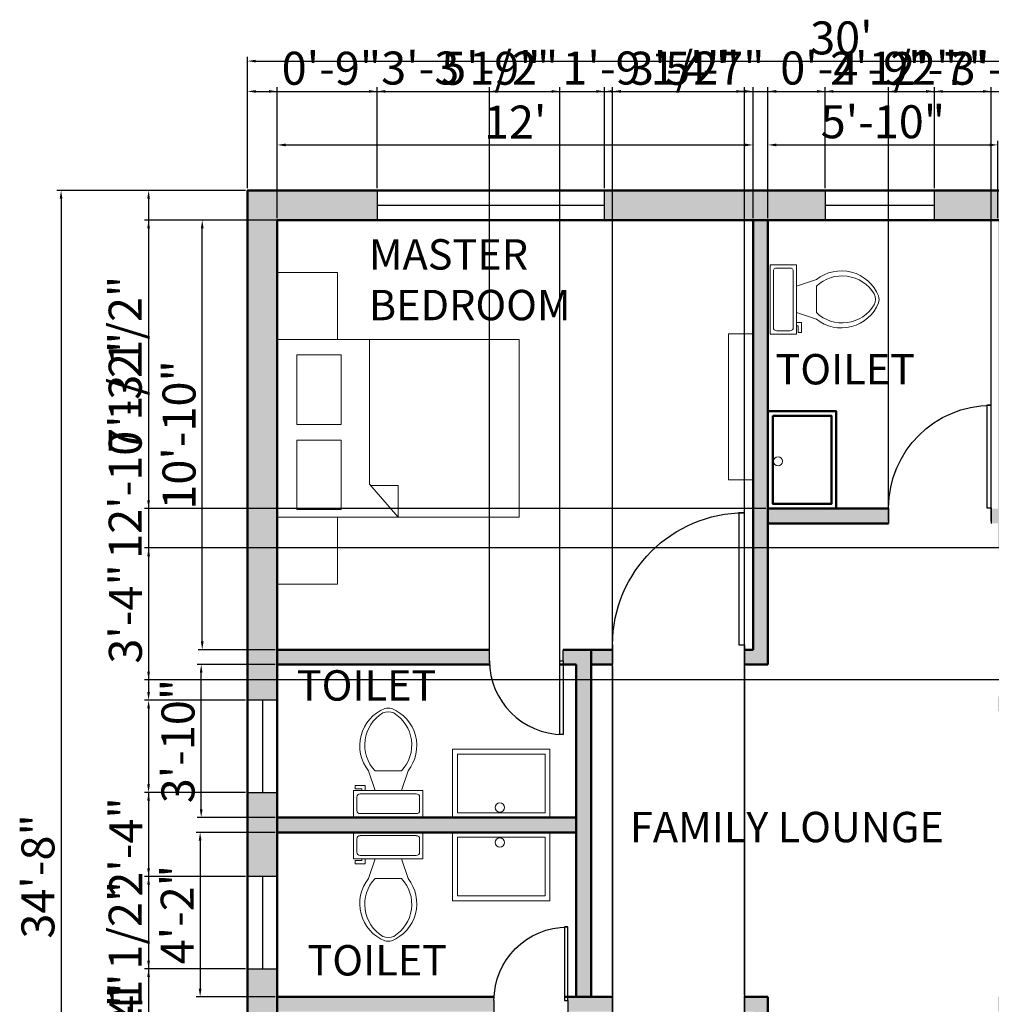
# Model space of a CAD drawing. Units: inches. Extents: x 1344 to 2521, y 3236 to 4924.
# Tile 2 of 14: x 1344 to 1639, y 3517 to 3815. Entities that reach past the tile are written whole.
import ezdxf

# ---------------------------------------------------------------- set-up
doc = ezdxf.new("R2010")
doc.units = ezdxf.units.IN
for name, color, linetype, lineweight in [('A-ANNO-DIMS', 2, 'Continuous', 18), ('A-AREA-IDEN', 3, 'Continuous', 18), ('A-DOOR', 50, 'Continuous', 25), ('A-FLOR-FIXT', 8, 'Continuous', 18), ('A-FURN', 130, 'Continuous', 18), ('A-GLAZ', 150, 'Continuous', 25), ('A-WALL', 31, 'Continuous', 50), ('A-WALL-PATT', 8, 'Continuous', 13)]:
    doc.layers.add(name, color=color, linetype=linetype, lineweight=lineweight)
doc.styles.get("Standard").update_dxf_attribs({"font": 'arial.ttf'})
doc.dimstyles.new('ISO-25', dxfattribs={"dimtxt": 10, "dimasz": 2.5, "dimexe": 1.25, "dimexo": 0.625, "dimtad": 1, "dimdec": 0, "dimlunit": 4, "dimtxsty": 'Standard', "dimcen": 2.5, "dimadec": 0, "dimazin": 0, "dimtfac": 1, "dimtdec": 0, "dimtmove": 0, "dimatfit": 3, "dimfxl": 1, "dimarcsym": 0})

# ---------------------------------------------------------------- blocks, each defined once
blk = doc.blocks.new('*U2')
for p, q in [((0, 0), (0, -6)), ((40, 0), (40, -6))]:
    blk.add_line(p, q)
blk.add_lwpolyline([(0, 0), (0, 40), (1.75, 40), (1.75, 0)], close=True)
blk.add_arc((0, 0), 40, 0, 90)
blk = doc.blocks.new('*U6')
for p, q in [((9.5, -6), (9.5, -2)), ((-10, -8.5), (-8, -8.5)), ((-10, -9.5), (-10, -8.5)), ((-8, -8.5), (-8, -8)), ((-7, -8), (-7, -9.5)), ((-4, -8), (-6, -14)), ((4, -8), (6, -14)), ((-7, -9.5), (-10, -9.5)), ((4, -14), (-4, -14))]:
    blk.add_line(p, q)
blk.add_lwpolyline([(10.5, -8), (10.5, 0), (-10.5, 0), (-10.5, -8)], close=True)
for points in [[(-9.5, -2), (-9.5, -6)], [(8.5, -1), (-8.5, -1)], [(-8.5, -7), (8.5, -7)]]:
    blk.add_lwpolyline(points)
for centre, radius, start, end in [((-8.62, -1.88), 0.884, 81.8699, 188.1301), ((8.62, -1.88), 0.884, 351.8699, 98.1301), ((-8.62, -6.12), 0.884, 171.8699, 278.1301), ((8.62, -6.12), 0.884, 261.8699, 8.1301), ((3.52, -21.58), 12.17, 141.4691, 247.9714), ((4.2, -21.82), 11.33, 136.3677, 238.9468), ((-3.52, -21.58), 12.17, 292.0284, 38.5307), ((-4.2, -21.82), 11.33, 301.053, 43.6321), ((0, -27.88), 4, 245.7318, 294.2682), ((0, -29), 4, 254.8605, 285.1395)]:
    blk.add_arc(centre, radius, start, end)
blk = doc.blocks.new('*D32')
at = {"layer": 'A-ANNO-DIMS', "color": 0, "lineweight": -2, "transparency": 16777216}
for p, q in [((1413.52, 3764.06), (1413.52, 3803.88)), ((1773.52, 3764.06), (1773.52, 3803.88)), ((1416.02, 3802.63), (1771.02, 3802.63))]:
    blk.add_line(p, q, dxfattribs=at)
at = {"layer": 'A-ANNO-DIMS', "color": 0, "lineweight": 100, "transparency": 16777216}
for points in [[(1416.02, 3803.04), (1416.02, 3802.21), (1413.52, 3802.63)], [(1771.02, 3803.04), (1771.02, 3802.21), (1773.52, 3802.63)]]:
    blk.add_solid(points, dxfattribs=at)
at = {"layer": 'Defpoints', "color": 0, "lineweight": 100, "transparency": 16777216}
for p in [(1773.52, 3802.63), (1413.52, 3763.43), (1773.52, 3763.43)]:
    blk.add_point(p, dxfattribs=at)
at = {"layer": 'A-ANNO-DIMS', "color": 0, "transparency": 16777216, "insert": (1593.52, 3808.36), "char_height": 10, "attachment_point": 5}
blk.add_mtext("30'", dxfattribs=at)
blk = doc.blocks.new('*D33')
at = {"layer": 'A-ANNO-DIMS', "color": 0, "lineweight": -2, "transparency": 16777216}
for p, q in [((1422.52, 3755.06), (1422.52, 3778.46)), ((1425.02, 3777.21), (1564.25, 3777.21)), ((1566.75, 3755.06), (1566.75, 3778.46))]:
    blk.add_line(p, q, dxfattribs=at)
at = {"layer": 'A-ANNO-DIMS', "color": 0, "lineweight": 100, "transparency": 16777216}
for points in [[(1425.02, 3777.62), (1425.02, 3776.79), (1422.52, 3777.21)], [(1564.25, 3777.62), (1564.25, 3776.79), (1566.75, 3777.21)]]:
    blk.add_solid(points, dxfattribs=at)
at = {"layer": 'Defpoints', "color": 0, "lineweight": 100, "transparency": 16777216}
for p in [(1566.75, 3777.21), (1422.52, 3754.43), (1566.75, 3754.43)]:
    blk.add_point(p, dxfattribs=at)
at = {"layer": 'A-ANNO-DIMS', "color": 0, "transparency": 16777216, "insert": (1494.63, 3782.85), "char_height": 10, "attachment_point": 5}
blk.add_mtext("12'", dxfattribs=at)
blk = doc.blocks.new('*D34')
at = {"layer": 'A-ANNO-DIMS', "color": 0, "lineweight": -2, "transparency": 16777216}
for p, q in [((1571.25, 3755.06), (1571.25, 3778.46)), ((1573.75, 3777.21), (1638.44, 3777.21)), ((1640.94, 3755.06), (1640.94, 3778.46))]:
    blk.add_line(p, q, dxfattribs=at)
at = {"layer": 'A-ANNO-DIMS', "color": 0, "lineweight": 100, "transparency": 16777216}
for points in [[(1573.75, 3777.62), (1573.75, 3776.79), (1571.25, 3777.21)], [(1638.44, 3777.62), (1638.44, 3776.79), (1640.94, 3777.21)]]:
    blk.add_solid(points, dxfattribs=at)
at = {"layer": 'Defpoints', "color": 0, "lineweight": 100, "transparency": 16777216}
for p in [(1640.94, 3777.21), (1571.25, 3754.43), (1640.94, 3754.43)]:
    blk.add_point(p, dxfattribs=at)
at = {"layer": 'A-ANNO-DIMS', "color": 0, "transparency": 16777216, "insert": (1606.1, 3782.94), "char_height": 10, "attachment_point": 5}
blk.add_mtext('5\'-10"', dxfattribs=at)
blk = doc.blocks.new('*D36')
at = {"layer": 'A-ANNO-DIMS', "color": 0, "lineweight": -2, "transparency": 16777216}
for p, q in [((1412.89, 3763.43), (1355.74, 3763.43)), ((1356.99, 3760.93), (1356.99, 3350.01)), ((1412.89, 3347.51), (1355.74, 3347.51))]:
    blk.add_line(p, q, dxfattribs=at)
at = {"layer": 'A-ANNO-DIMS', "color": 0, "lineweight": 100, "transparency": 16777216}
for points in [[(1356.58, 3760.93), (1357.41, 3760.93), (1356.99, 3763.43)], [(1356.58, 3350.01), (1357.41, 3350.01), (1356.99, 3347.51)]]:
    blk.add_solid(points, dxfattribs=at)
at = {"layer": 'Defpoints', "color": 0, "lineweight": 100, "transparency": 16777216}
for p in [(1413.52, 3763.43), (1356.99, 3347.51), (1413.52, 3347.51)]:
    blk.add_point(p, dxfattribs=at)
at = {"layer": 'A-ANNO-DIMS', "color": 0, "transparency": 16777216, "insert": (1351.26, 3555.47), "char_height": 10, "attachment_point": 5, "rotation": 90}
blk.add_mtext('34\'-8"', dxfattribs=at)
blk = doc.blocks.new('*D44')
at = {"layer": 'A-ANNO-DIMS', "color": 0, "lineweight": -2, "transparency": 16777216}
for p, q in [((1421.89, 3754.43), (1398.53, 3754.43)), ((1399.78, 3626.69), (1399.78, 3751.93)), ((1421.89, 3624.19), (1398.53, 3624.19))]:
    blk.add_line(p, q, dxfattribs=at)
at = {"layer": 'A-ANNO-DIMS', "color": 0, "lineweight": 100, "transparency": 16777216}
for points in [[(1399.36, 3751.93), (1400.19, 3751.93), (1399.78, 3754.43)], [(1399.36, 3626.69), (1400.19, 3626.69), (1399.78, 3624.19)]]:
    blk.add_solid(points, dxfattribs=at)
at = {"layer": 'Defpoints', "color": 0, "lineweight": 100, "transparency": 16777216}
for p in [(1399.78, 3754.43), (1422.52, 3754.43), (1422.52, 3624.19)]:
    blk.add_point(p, dxfattribs=at)
at = {"layer": 'A-ANNO-DIMS', "color": 0, "transparency": 16777216, "insert": (1394.04, 3689.31), "char_height": 10, "attachment_point": 5, "rotation": 90}
blk.add_mtext('10\'-10"', dxfattribs=at)
blk = doc.blocks.new('*D45')
at = {"layer": 'A-ANNO-DIMS', "color": 0, "lineweight": -2, "transparency": 16777216}
for p, q in [((1421.89, 3619.69), (1398.21, 3619.69)), ((1399.46, 3575.82), (1399.46, 3617.19)), ((1421.89, 3573.32), (1398.21, 3573.32))]:
    blk.add_line(p, q, dxfattribs=at)
at = {"layer": 'A-ANNO-DIMS', "color": 0, "lineweight": 100, "transparency": 16777216}
for points in [[(1399.04, 3617.19), (1399.87, 3617.19), (1399.46, 3619.69)], [(1399.04, 3575.82), (1399.87, 3575.82), (1399.46, 3573.32)]]:
    blk.add_solid(points, dxfattribs=at)
at = {"layer": 'Defpoints', "color": 0, "lineweight": 100, "transparency": 16777216}
for p in [(1399.46, 3619.69), (1422.52, 3619.69), (1422.52, 3573.32)]:
    blk.add_point(p, dxfattribs=at)
at = {"layer": 'A-ANNO-DIMS', "color": 0, "transparency": 16777216, "insert": (1393.72, 3596.5), "char_height": 10, "attachment_point": 5, "rotation": 90}
blk.add_mtext('3\'-10"', dxfattribs=at)
blk = doc.blocks.new('*D46')
at = {"layer": 'A-ANNO-DIMS', "color": 0, "lineweight": -2, "transparency": 16777216}
for p, q in [((1421.89, 3568.82), (1397.89, 3568.82)), ((1399.14, 3566.32), (1399.14, 3521.45)), ((1421.89, 3518.95), (1397.89, 3518.95))]:
    blk.add_line(p, q, dxfattribs=at)
at = {"layer": 'A-ANNO-DIMS', "color": 0, "lineweight": 100, "transparency": 16777216}
for points in [[(1398.72, 3566.32), (1399.55, 3566.32), (1399.14, 3568.82)], [(1398.72, 3521.45), (1399.55, 3521.45), (1399.14, 3518.95)]]:
    blk.add_solid(points, dxfattribs=at)
at = {"layer": 'Defpoints', "color": 0, "lineweight": 100, "transparency": 16777216}
for p in [(1422.52, 3568.82), (1399.14, 3518.95), (1422.52, 3518.95)]:
    blk.add_point(p, dxfattribs=at)
at = {"layer": 'A-ANNO-DIMS', "color": 0, "transparency": 16777216, "insert": (1393.49, 3543.88), "char_height": 10, "attachment_point": 5, "rotation": 90}
blk.add_mtext('4\'-2"', dxfattribs=at)
blk = doc.blocks.new('BED-DOUBLE')
for p, q in [((27.95, 53.78), (27.95, 9.98)), ((27.95, 9.98), (36.68, 0)), ((36.68, 9.56), (28.32, 9.56)), ((36.68, 0), (36.68, 9.56))]:
    blk.add_line(p, q)
for points in [[(0, 0), (73.35, 0), (73.35, 53.78), (0, 53.78)], [(5.91, 28.08), (19.39, 28.08), (19.39, 49.13), (5.91, 49.13)], [(5.91, 2.27), (19.39, 2.27), (19.39, 23.31), (5.91, 23.31)]]:
    blk.add_lwpolyline(points, close=True)
blk = doc.blocks.new('WASH-BASIN')
for points in [[(29.51, 20.73), (0, 20.73), (0, 0), (29.51, 0)], [(28.05, 19.27), (1.46, 19.27), (1.46, 1.46), (28.05, 1.46)]]:
    blk.add_lwpolyline(points, close=True)
blk.add_circle((14.31, 17.66), 1.38)
blk = doc.blocks.new('*D153')
at = {"layer": 'A-ANNO-DIMS', "color": 0, "lineweight": -2, "transparency": 16777216}
for p, q in [((1413.52, 3764.06), (1413.52, 3794.68)), ((1422.52, 3755.06), (1422.52, 3794.68)), ((1416.02, 3793.43), (1420.02, 3793.43)), ((1422.52, 3793.43), (1452.85, 3793.43))]:
    blk.add_line(p, q, dxfattribs=at)
at = {"layer": 'A-ANNO-DIMS', "color": 0, "lineweight": 100, "transparency": 16777216}
for points in [[(1416.02, 3793.85), (1416.02, 3793.02), (1413.52, 3793.43)], [(1420.02, 3793.85), (1420.02, 3793.02), (1422.52, 3793.43)]]:
    blk.add_solid(points, dxfattribs=at)
at = {"layer": 'Defpoints', "color": 0, "lineweight": 100, "transparency": 16777216}
for p in [(1422.52, 3793.43), (1413.52, 3763.43), (1422.52, 3754.43)]:
    blk.add_point(p, dxfattribs=at)
at = {"layer": 'A-ANNO-DIMS', "color": 0, "transparency": 16777216, "insert": (1438.93, 3799.16), "char_height": 10, "attachment_point": 5}
blk.add_mtext('0\'-9"', dxfattribs=at)
blk = doc.blocks.new('*D154')
at = {"layer": 'A-ANNO-DIMS', "color": 0, "lineweight": -2, "transparency": 16777216}
for p, q in [((1566.75, 3755.06), (1566.75, 3794.68)), ((1571.25, 3755.06), (1571.25, 3794.68)), ((1564.25, 3793.43), (1561.75, 3793.43)), ((1566.75, 3793.43), (1571.25, 3793.43)), ((1573.75, 3793.43), (1627.39, 3793.43))]:
    blk.add_line(p, q, dxfattribs=at)
at = {"layer": 'A-ANNO-DIMS', "color": 0, "lineweight": 100, "transparency": 16777216}
for points in [[(1564.25, 3793.85), (1564.25, 3793.02), (1566.75, 3793.43)], [(1573.75, 3793.85), (1573.75, 3793.02), (1571.25, 3793.43)]]:
    blk.add_solid(points, dxfattribs=at)
at = {"layer": 'Defpoints', "color": 0, "lineweight": 100, "transparency": 16777216}
for p in [(1571.25, 3793.43), (1566.75, 3754.43), (1571.25, 3754.43)]:
    blk.add_point(p, dxfattribs=at)
at = {"layer": 'A-ANNO-DIMS', "color": 0, "transparency": 16777216, "insert": (1601.82, 3799.23), "char_height": 10, "attachment_point": 5}
blk.add_mtext('0\'-4 1/2"', dxfattribs=at)
blk = doc.blocks.new('*D155')
at = {"layer": 'A-ANNO-DIMS', "color": 0, "lineweight": -2, "transparency": 16777216}
for p, q in [((1413.52, 3764.06), (1413.52, 3794.68)), ((1452.8, 3764.06), (1452.8, 3794.68)), ((1416.02, 3793.43), (1450.3, 3793.43)), ((1452.8, 3793.43), (1506.43, 3793.43))]:
    blk.add_line(p, q, dxfattribs=at)
at = {"layer": 'A-ANNO-DIMS', "color": 0, "lineweight": 100, "transparency": 16777216}
for points in [[(1416.02, 3793.85), (1416.02, 3793.02), (1413.52, 3793.43)], [(1450.3, 3793.85), (1450.3, 3793.02), (1452.8, 3793.43)]]:
    blk.add_solid(points, dxfattribs=at)
at = {"layer": 'Defpoints', "color": 0, "lineweight": 100, "transparency": 16777216}
for p in [(1452.8, 3793.43), (1413.52, 3763.43), (1452.8, 3763.43)]:
    blk.add_point(p, dxfattribs=at)
at = {"layer": 'A-ANNO-DIMS', "color": 0, "transparency": 16777216, "insert": (1480.86, 3799.23), "char_height": 10, "attachment_point": 5}
blk.add_mtext('3\'-3 1/2"', dxfattribs=at)
blk = doc.blocks.new('*D156')
at = {"layer": 'A-ANNO-DIMS', "color": 0, "lineweight": -2, "transparency": 16777216}
for p, q in [((1452.8, 3764.06), (1452.8, 3794.68)), ((1521.72, 3764.06), (1521.72, 3794.68)), ((1455.3, 3793.43), (1519.22, 3793.43))]:
    blk.add_line(p, q, dxfattribs=at)
at = {"layer": 'A-ANNO-DIMS', "color": 0, "lineweight": 100, "transparency": 16777216}
for points in [[(1455.3, 3793.85), (1455.3, 3793.02), (1452.8, 3793.43)], [(1519.22, 3793.85), (1519.22, 3793.02), (1521.72, 3793.43)]]:
    blk.add_solid(points, dxfattribs=at)
at = {"layer": 'Defpoints', "color": 0, "lineweight": 100, "transparency": 16777216}
for p in [(1521.72, 3793.43), (1452.8, 3763.43), (1521.72, 3763.43)]:
    blk.add_point(p, dxfattribs=at)
at = {"layer": 'A-ANNO-DIMS', "color": 0, "transparency": 16777216, "insert": (1487.26, 3799.16), "char_height": 10, "attachment_point": 5}
blk.add_mtext('5\'-9"', dxfattribs=at)
blk = doc.blocks.new('*D157')
at = {"layer": 'A-ANNO-DIMS', "color": 0, "lineweight": -2, "transparency": 16777216}
for p, q in [((1521.72, 3764.06), (1521.72, 3794.68)), ((1588.61, 3764.06), (1588.61, 3794.68)), ((1524.22, 3793.43), (1586.11, 3793.43))]:
    blk.add_line(p, q, dxfattribs=at)
at = {"layer": 'A-ANNO-DIMS', "color": 0, "lineweight": 100, "transparency": 16777216}
for points in [[(1524.22, 3793.85), (1524.22, 3793.02), (1521.72, 3793.43)], [(1586.11, 3793.85), (1586.11, 3793.02), (1588.61, 3793.43)]]:
    blk.add_solid(points, dxfattribs=at)
at = {"layer": 'Defpoints', "color": 0, "lineweight": 100, "transparency": 16777216}
for p in [(1588.61, 3793.43), (1521.72, 3763.43), (1588.61, 3763.43)]:
    blk.add_point(p, dxfattribs=at)
at = {"layer": 'A-ANNO-DIMS', "color": 0, "transparency": 16777216, "insert": (1555.17, 3799.14), "char_height": 10, "attachment_point": 5}
blk.add_mtext('5\'-7"', dxfattribs=at)
blk = doc.blocks.new('*D158')
at = {"layer": 'A-ANNO-DIMS', "color": 0, "lineweight": -2, "transparency": 16777216}
for p, q in [((1588.61, 3764.06), (1588.61, 3794.68)), ((1621.71, 3764.06), (1621.71, 3794.68)), ((1591.11, 3793.43), (1619.21, 3793.43))]:
    blk.add_line(p, q, dxfattribs=at)
at = {"layer": 'A-ANNO-DIMS', "color": 0, "lineweight": 100, "transparency": 16777216}
for points in [[(1591.11, 3793.85), (1591.11, 3793.02), (1588.61, 3793.43)], [(1619.21, 3793.85), (1619.21, 3793.02), (1621.71, 3793.43)]]:
    blk.add_solid(points, dxfattribs=at)
at = {"layer": 'Defpoints', "color": 0, "lineweight": 100, "transparency": 16777216}
for p in [(1621.71, 3793.43), (1588.61, 3763.43), (1621.71, 3763.43)]:
    blk.add_point(p, dxfattribs=at)
at = {"layer": 'A-ANNO-DIMS', "color": 0, "transparency": 16777216, "insert": (1605.16, 3799.16), "char_height": 10, "attachment_point": 5}
blk.add_mtext('2\'-9"', dxfattribs=at)
blk = doc.blocks.new('*D159')
at = {"layer": 'A-ANNO-DIMS', "color": 0, "lineweight": -2, "transparency": 16777216}
for p, q in [((1621.71, 3764.06), (1621.71, 3794.68)), ((1661.64, 3764.06), (1661.64, 3794.68)), ((1624.21, 3793.43), (1659.14, 3793.43))]:
    blk.add_line(p, q, dxfattribs=at)
at = {"layer": 'A-ANNO-DIMS', "color": 0, "lineweight": 100, "transparency": 16777216}
for points in [[(1624.21, 3793.85), (1624.21, 3793.02), (1621.71, 3793.43)], [(1659.14, 3793.85), (1659.14, 3793.02), (1661.64, 3793.43)]]:
    blk.add_solid(points, dxfattribs=at)
at = {"layer": 'Defpoints', "color": 0, "lineweight": 100, "transparency": 16777216}
for p in [(1661.64, 3793.43), (1621.71, 3763.43), (1661.64, 3763.43)]:
    blk.add_point(p, dxfattribs=at)
at = {"layer": 'A-ANNO-DIMS', "color": 0, "transparency": 16777216, "insert": (1641.68, 3799.17), "char_height": 10, "attachment_point": 5}
blk.add_mtext('3\'-4"', dxfattribs=at)
blk = doc.blocks.new('*D162')
at = {"layer": 'A-ANNO-DIMS', "color": 0, "lineweight": -2, "transparency": 16777216}
for p, q in [((1412.89, 3763.43), (1382.27, 3763.43)), ((1383.52, 3760.93), (1383.52, 3611.37)), ((1412.89, 3608.87), (1382.27, 3608.87))]:
    blk.add_line(p, q, dxfattribs=at)
at = {"layer": 'A-ANNO-DIMS', "color": 0, "lineweight": 100, "transparency": 16777216}
for points in [[(1383.1, 3760.93), (1383.93, 3760.93), (1383.52, 3763.43)], [(1383.1, 3611.37), (1383.93, 3611.37), (1383.52, 3608.87)]]:
    blk.add_solid(points, dxfattribs=at)
at = {"layer": 'Defpoints', "color": 0, "lineweight": 100, "transparency": 16777216}
for p in [(1413.52, 3763.43), (1383.52, 3608.87), (1413.52, 3608.87)]:
    blk.add_point(p, dxfattribs=at)
at = {"layer": 'A-ANNO-DIMS', "color": 0, "transparency": 16777216, "insert": (1377.72, 3686.15), "char_height": 10, "attachment_point": 5, "rotation": 90}
blk.add_mtext('12\'-10 1/2"', dxfattribs=at)
blk = doc.blocks.new('*D163')
at = {"layer": 'A-ANNO-DIMS', "color": 0, "lineweight": -2, "transparency": 16777216}
for p, q in [((1412.89, 3608.87), (1382.27, 3608.87)), ((1383.52, 3606.37), (1383.52, 3583.39)), ((1412.89, 3580.89), (1382.27, 3580.89)), ((1383.52, 3580.89), (1383.52, 3550.39))]:
    blk.add_line(p, q, dxfattribs=at)
at = {"layer": 'A-ANNO-DIMS', "color": 0, "lineweight": 100, "transparency": 16777216}
for points in [[(1383.1, 3606.37), (1383.93, 3606.37), (1383.52, 3608.87)], [(1383.1, 3583.39), (1383.93, 3583.39), (1383.52, 3580.89)]]:
    blk.add_solid(points, dxfattribs=at)
at = {"layer": 'Defpoints', "color": 0, "lineweight": 100, "transparency": 16777216}
for p in [(1413.52, 3608.87), (1383.52, 3580.89), (1413.52, 3580.89)]:
    blk.add_point(p, dxfattribs=at)
at = {"layer": 'A-ANNO-DIMS', "color": 0, "transparency": 16777216, "insert": (1377.87, 3564.39), "char_height": 10, "attachment_point": 5, "rotation": 90}
blk.add_mtext('2\'-4"', dxfattribs=at)
blk = doc.blocks.new('*D164')
at = {"layer": 'A-ANNO-DIMS', "color": 0, "lineweight": -2, "transparency": 16777216}
for p, q in [((1412.89, 3580.89), (1382.27, 3580.89)), ((1383.52, 3578.39), (1383.52, 3557.95)), ((1412.89, 3555.45), (1382.27, 3555.45)), ((1383.52, 3555.45), (1383.52, 3501.65))]:
    blk.add_line(p, q, dxfattribs=at)
at = {"layer": 'A-ANNO-DIMS', "color": 0, "lineweight": 100, "transparency": 16777216}
for points in [[(1383.1, 3578.39), (1383.93, 3578.39), (1383.52, 3580.89)], [(1383.1, 3557.95), (1383.93, 3557.95), (1383.52, 3555.45)]]:
    blk.add_solid(points, dxfattribs=at)
at = {"layer": 'Defpoints', "color": 0, "lineweight": 100, "transparency": 16777216}
for p in [(1413.52, 3580.89), (1383.52, 3555.45), (1413.52, 3555.45)]:
    blk.add_point(p, dxfattribs=at)
at = {"layer": 'A-ANNO-DIMS', "color": 0, "transparency": 16777216, "insert": (1377.72, 3527.3), "char_height": 10, "attachment_point": 5, "rotation": 90}
blk.add_mtext('2\'-1 1/2"', dxfattribs=at)
blk = doc.blocks.new('*D165')
at = {"layer": 'A-ANNO-DIMS', "color": 0, "lineweight": -2, "transparency": 16777216}
for p, q in [((1412.89, 3555.45), (1382.27, 3555.45)), ((1383.52, 3552.95), (1383.52, 3529.97)), ((1412.89, 3527.47), (1382.27, 3527.47)), ((1383.52, 3527.47), (1383.52, 3496.97))]:
    blk.add_line(p, q, dxfattribs=at)
at = {"layer": 'A-ANNO-DIMS', "color": 0, "lineweight": 100, "transparency": 16777216}
for points in [[(1383.1, 3552.95), (1383.93, 3552.95), (1383.52, 3555.45)], [(1383.1, 3529.97), (1383.93, 3529.97), (1383.52, 3527.47)]]:
    blk.add_solid(points, dxfattribs=at)
at = {"layer": 'Defpoints', "color": 0, "lineweight": 100, "transparency": 16777216}
for p in [(1413.52, 3555.45), (1383.52, 3527.47), (1413.52, 3527.47)]:
    blk.add_point(p, dxfattribs=at)
at = {"layer": 'A-ANNO-DIMS', "color": 0, "transparency": 16777216, "insert": (1377.87, 3510.97), "char_height": 10, "attachment_point": 5, "rotation": 90}
blk.add_mtext('2\'-4"', dxfattribs=at)
blk = doc.blocks.new('*D166')
at = {"layer": 'A-ANNO-DIMS', "color": 0, "lineweight": -2, "transparency": 16777216}
for p, q in [((1412.89, 3527.47), (1382.27, 3527.47)), ((1383.52, 3524.97), (1383.52, 3458.32)), ((1412.89, 3455.82), (1382.27, 3455.82))]:
    blk.add_line(p, q, dxfattribs=at)
at = {"layer": 'A-ANNO-DIMS', "color": 0, "lineweight": 100, "transparency": 16777216}
for points in [[(1383.1, 3524.97), (1383.93, 3524.97), (1383.52, 3527.47)], [(1383.1, 3458.32), (1383.93, 3458.32), (1383.52, 3455.82)]]:
    blk.add_solid(points, dxfattribs=at)
at = {"layer": 'Defpoints', "color": 0, "lineweight": 100, "transparency": 16777216}
for p in [(1413.52, 3527.47), (1383.52, 3455.82), (1413.52, 3455.82)]:
    blk.add_point(p, dxfattribs=at)
at = {"layer": 'A-ANNO-DIMS', "color": 0, "transparency": 16777216, "insert": (1377.72, 3491.65), "char_height": 10, "attachment_point": 5, "rotation": 90}
blk.add_mtext('5\'-11 1/2"', dxfattribs=at)
blk = doc.blocks.new('*D174')
at = {"layer": 'A-ANNO-DIMS', "color": 0, "lineweight": -2, "transparency": 16777216}
for p, q in [((1486.87, 3620.31), (1486.87, 3794.68)), ((1508.2, 3620.31), (1508.2, 3794.68)), ((1489.37, 3793.43), (1505.7, 3793.43)), ((1508.2, 3793.43), (1560.89, 3793.43))]:
    blk.add_line(p, q, dxfattribs=at)
at = {"layer": 'A-ANNO-DIMS', "color": 0, "lineweight": 100, "transparency": 16777216}
for points in [[(1489.37, 3793.85), (1489.37, 3793.02), (1486.87, 3793.43)], [(1505.7, 3793.85), (1505.7, 3793.02), (1508.2, 3793.43)]]:
    blk.add_solid(points, dxfattribs=at)
at = {"layer": 'Defpoints', "color": 0, "lineweight": 100, "transparency": 16777216}
for p in [(1508.2, 3793.43), (1486.87, 3619.69), (1508.2, 3619.69)]:
    blk.add_point(p, dxfattribs=at)
at = {"layer": 'A-ANNO-DIMS', "color": 0, "transparency": 16777216, "insert": (1535.8, 3799.23), "char_height": 10, "attachment_point": 5}
blk.add_mtext('1\'-9 1/2"', dxfattribs=at)
blk = doc.blocks.new('*D175')
at = {"layer": 'A-ANNO-DIMS', "color": 0, "lineweight": -2, "transparency": 16777216}
for p, q in [((1524.17, 3619.06), (1524.17, 3316.22)), ((1564.17, 3619.06), (1564.17, 3316.22)), ((1526.67, 3317.47), (1561.67, 3317.47))]:
    blk.add_line(p, q, dxfattribs=at)
at = {"layer": 'A-ANNO-DIMS', "color": 0, "lineweight": 100, "transparency": 16777216}
for points in [[(1526.67, 3317.89), (1526.67, 3317.06), (1524.17, 3317.47)], [(1561.67, 3317.89), (1561.67, 3317.06), (1564.17, 3317.47)]]:
    blk.add_solid(points, dxfattribs=at)
at = {"layer": 'Defpoints', "color": 0, "lineweight": 100, "transparency": 16777216}
for p in [(1524.17, 3619.69), (1564.17, 3619.69), (1564.17, 3317.47)]:
    blk.add_point(p, dxfattribs=at)
at = {"layer": 'A-ANNO-DIMS', "color": 0, "transparency": 16777216, "insert": (1544.17, 3323.21), "char_height": 10, "attachment_point": 5}
blk.add_mtext('3\'-4"', dxfattribs=at)
blk = doc.blocks.new('*D177')
at = {"layer": 'A-ANNO-DIMS', "color": 0, "lineweight": -2, "transparency": 16777216}
for p, q in [((1524.17, 3519.57), (1524.17, 3794.68)), ((1564.17, 3519.57), (1564.17, 3794.68)), ((1526.67, 3793.43), (1561.67, 3793.43))]:
    blk.add_line(p, q, dxfattribs=at)
at = {"layer": 'A-ANNO-DIMS', "color": 0, "lineweight": 100, "transparency": 16777216}
for points in [[(1526.67, 3793.85), (1526.67, 3793.02), (1524.17, 3793.43)], [(1561.67, 3793.85), (1561.67, 3793.02), (1564.17, 3793.43)]]:
    blk.add_solid(points, dxfattribs=at)
at = {"layer": 'Defpoints', "color": 0, "lineweight": 100, "transparency": 16777216}
for p in [(1564.17, 3793.43), (1524.17, 3518.95), (1564.17, 3518.95)]:
    blk.add_point(p, dxfattribs=at)
at = {"layer": 'A-ANNO-DIMS', "color": 0, "transparency": 16777216, "insert": (1544.17, 3799.17), "char_height": 10, "attachment_point": 5}
blk.add_mtext('3\'-4"', dxfattribs=at)
blk = doc.blocks.new('*D178')
at = {"layer": 'A-ANNO-DIMS', "color": 0, "lineweight": -2, "transparency": 16777216}
for p, q in [((1570.63, 3754.43), (1382.27, 3754.43)), ((1383.52, 3751.93), (1383.52, 3669.49)), ((1570.63, 3666.99), (1382.27, 3666.99))]:
    blk.add_line(p, q, dxfattribs=at)
at = {"layer": 'A-ANNO-DIMS', "color": 0, "lineweight": 100, "transparency": 16777216}
for points in [[(1383.1, 3751.93), (1383.93, 3751.93), (1383.52, 3754.43)], [(1383.1, 3669.49), (1383.93, 3669.49), (1383.52, 3666.99)]]:
    blk.add_solid(points, dxfattribs=at)
at = {"layer": 'Defpoints', "color": 0, "lineweight": 100, "transparency": 16777216}
for p in [(1571.25, 3754.43), (1383.52, 3666.99), (1571.25, 3666.99)]:
    blk.add_point(p, dxfattribs=at)
at = {"layer": 'A-ANNO-DIMS', "color": 0, "transparency": 16777216, "insert": (1377.72, 3710.71), "char_height": 10, "attachment_point": 5, "rotation": 90}
blk.add_mtext('7\'-3 1/2"', dxfattribs=at)
blk = doc.blocks.new('*D179')
at = {"layer": 'A-ANNO-DIMS', "color": 0, "lineweight": -2, "transparency": 16777216}
for p, q in [((1607.83, 3663.12), (1607.83, 3794.68)), ((1638.96, 3663.12), (1638.96, 3794.68)), ((1610.33, 3793.43), (1636.46, 3793.43))]:
    blk.add_line(p, q, dxfattribs=at)
at = {"layer": 'A-ANNO-DIMS', "color": 0, "lineweight": 100, "transparency": 16777216}
for points in [[(1610.33, 3793.85), (1610.33, 3793.02), (1607.83, 3793.43)], [(1636.46, 3793.85), (1636.46, 3793.02), (1638.96, 3793.43)]]:
    blk.add_solid(points, dxfattribs=at)
at = {"layer": 'Defpoints', "color": 0, "lineweight": 100, "transparency": 16777216}
for p in [(1638.96, 3793.43), (1607.83, 3662.49), (1638.96, 3662.49)]:
    blk.add_point(p, dxfattribs=at)
at = {"layer": 'A-ANNO-DIMS', "color": 0, "transparency": 16777216, "insert": (1623.39, 3799.08), "char_height": 10, "attachment_point": 5}
blk.add_mtext('2\'-7"', dxfattribs=at)
blk = doc.blocks.new('*D180')
at = {"layer": 'A-ANNO-DIMS', "color": 0, "lineweight": -2, "transparency": 16777216}
for p, q in [((1644.82, 3655.04), (1382.27, 3655.04)), ((1383.52, 3652.54), (1383.52, 3617.54)), ((1644.82, 3615.04), (1382.27, 3615.04))]:
    blk.add_line(p, q, dxfattribs=at)
at = {"layer": 'A-ANNO-DIMS', "color": 0, "lineweight": 100, "transparency": 16777216}
for points in [[(1383.1, 3652.54), (1383.93, 3652.54), (1383.52, 3655.04)], [(1383.1, 3617.54), (1383.93, 3617.54), (1383.52, 3615.04)]]:
    blk.add_solid(points, dxfattribs=at)
at = {"layer": 'Defpoints', "color": 0, "lineweight": 100, "transparency": 16777216}
for p in [(1645.44, 3655.04), (1383.52, 3615.04), (1645.44, 3615.04)]:
    blk.add_point(p, dxfattribs=at)
at = {"layer": 'A-ANNO-DIMS', "color": 0, "transparency": 16777216, "insert": (1377.78, 3635.04), "char_height": 10, "attachment_point": 5, "rotation": 90}
blk.add_mtext('3\'-4"', dxfattribs=at)

msp = doc.modelspace()

# ---------------------------------------------------------------- hatches: boundary and pattern name
at = {"layer": 'A-WALL-PATT'}
h = msp.add_hatch(color=256, dxfattribs=at)
h.dxf.hatch_style = 1
h.paths.add_polyline_path([(1452.8, 3763.43), (1413.52, 3763.43), (1413.52, 3608.87), (1422.52, 3608.87), (1422.52, 3754.43), (1452.8, 3754.43)])
h.paths.add_polyline_path([(1588.61, 3763.43), (1521.72, 3763.43), (1521.72, 3754.43), (1588.61, 3754.43)])
h.paths.add_polyline_path([(1661.64, 3763.43), (1621.71, 3763.43), (1621.71, 3754.43), (1661.64, 3754.43)])
h.paths.add_polyline_path([(1773.52, 3763.43), (1730.56, 3763.43), (1730.56, 3754.43), (1764.52, 3754.43), (1764.52, 3594.28), (1773.52, 3594.28)])
h.paths.add_polyline_path([(1645.44, 3754.43), (1640.94, 3754.43), (1640.94, 3655.04), (1645.44, 3655.04)])
h.paths.add_polyline_path([(1571.25, 3754.43), (1566.75, 3754.43), (1566.75, 3624.19), (1566.51, 3624.19), (1564.17, 3624.19), (1564.17, 3619.69), (1571.25, 3619.69)])
h.paths.add_polyline_path([(1607.83, 3666.99), (1571.25, 3666.99), (1571.25, 3662.49), (1607.83, 3662.49)])
h.paths.add_polyline_path([(1640.94, 3666.99), (1638.96, 3666.99), (1638.96, 3662.49), (1640.94, 3662.49)])
h.paths.add_polyline_path([(1524.17, 3624.19), (1517.67, 3624.19), (1517.67, 3619.69), (1524.17, 3619.69)])
h = msp.add_hatch(color=256, dxfattribs=at)
h.dxf.hatch_style = 1
h.paths.add_polyline_path([(1451.85, 3356.47), (1422.52, 3356.47), (1422.52, 3386.9), (1413.52, 3386.9), (1413.52, 3347.51), (1451.85, 3347.51)])
h.paths.add_polyline_path([(1744.16, 3352.01), (1566.75, 3352.01), (1566.75, 3356.47), (1544.82, 3356.47), (1520.77, 3356.47), (1520.77, 3347.51), (1744.16, 3347.51)])
h.paths.add_polyline_path([(1773.52, 3525.36), (1764.52, 3525.36), (1764.52, 3497.27), (1764.52, 3412.01), (1764.72, 3412.01), (1764.72, 3403.01), (1764.52, 3403.01), (1764.52, 3356.51), (1744.16, 3356.51), (1744.16, 3347.51), (1773.52, 3347.51)])
h.paths.add_polyline_path([(1764.52, 3412.01), (1740.62, 3412.01), (1740.62, 3403.01), (1764.52, 3403.01)])
h.paths.add_polyline_path([(1668.63, 3412.01), (1644.53, 3412.01), (1644.53, 3403.01), (1668.63, 3403.01)])
h.paths.add_polyline_path([(1571.25, 3514.45), (1571.25, 3518.95), (1564.17, 3518.95), (1564.17, 3514.45), (1566.75, 3514.45), (1566.75, 3352.01), (1571.25, 3352.01)])
h.paths.add_polyline_path([(1422.52, 3527.47), (1413.52, 3527.47), (1413.52, 3455.82), (1422.52, 3455.82), (1422.52, 3470.24)])
h.paths.add_polyline_path([(1488.21, 3517.8, -0.012876), (1488.24, 3518.95), (1422.52, 3518.95), (1422.52, 3514.45), (1488.21, 3514.45)])
h.paths.add_polyline_path([(1524.17, 3518.95), (1510.55, 3518.95), (1510.55, 3517.8), (1510.55, 3514.45), (1524.17, 3514.45)])
h.paths.add_polyline_path([(1764.52, 3518.95), (1640.94, 3518.95), (1640.94, 3514.45), (1764.52, 3514.45)])
h.paths.add_polyline_path([(1764.52, 3610.02), (1645.44, 3610.02), (1645.44, 3605.52), (1764.52, 3605.52)])
h.paths.add_polyline_path([(1645.44, 3610.02), (1640.94, 3610.02), (1640.94, 3605.52), (1645.44, 3605.52)])
h.paths.add_polyline_path([(1422.52, 3580.89), (1413.52, 3580.89), (1413.52, 3555.45), (1422.52, 3555.45)])
h.paths.add_polyline_path([(1513.17, 3573.32), (1505.17, 3573.32), (1505.17, 3573.28), (1475.67, 3573.28), (1422.52, 3573.32), (1422.52, 3568.82), (1513.17, 3568.82)])
h.paths.add_polyline_path([(1635.28, 3376.69), (1701.38, 3376.69), (1701.38, 3395.67), (1635.28, 3395.67)], flags=9)
h.paths.add_polyline_path([(1526.07, 3560.64), (1635.07, 3560.64), (1635.07, 3579.62), (1526.07, 3579.62)], flags=9)
h.paths.add_polyline_path([(1666.39, 3730.09), (1741.06, 3730.09), (1741.06, 3749.07), (1666.39, 3749.07)], flags=9)
h.paths.add_polyline_path([(1446.44, 3467.76), (1517.54, 3467.76), (1517.54, 3502.26), (1446.44, 3502.26)], flags=9)
h.paths.add_polyline_path([(1429.07, 3520.24), (1478.72, 3520.24), (1478.72, 3539.22), (1429.07, 3539.22)], flags=9)
h.paths.add_polyline_path([(1425.85, 3603.57), (1475.5, 3603.57), (1475.5, 3622.55), (1425.85, 3622.55)], flags=9)
h.paths.add_polyline_path([(1570.93, 3699.42), (1620.58, 3699.42), (1620.58, 3718.41), (1570.93, 3718.41)], flags=9)
h.paths.add_polyline_path([(1447.04, 3718.72), (1518.14, 3718.72), (1518.14, 3753.22), (1447.04, 3753.22)], flags=9)
h = msp.add_hatch(color=256, dxfattribs=at)
h.dxf.hatch_style = 1
h.paths.add_polyline_path([(1517.67, 3624.19), (1509.18, 3624.19), (1509.18, 3620.84), (1509.18, 3619.69), (1513.17, 3619.69), (1513.17, 3518.95), (1517.67, 3518.95)])
h.paths.add_polyline_path([(1486.84, 3624.19), (1422.52, 3624.19), (1422.52, 3619.69), (1486.87, 3619.69, -0.012876), (1486.84, 3620.84)])

# ---------------------------------------------------------------- linework, layer by layer
at = {"layer": 'A-FLOR-FIXT'}
msp.add_circle((1574.32, 3681.31), 1.38, dxfattribs=at)
at = {"layer": 'A-FURN'}
for points in [[(1422.52, 3718.19), (1440.75, 3718.19), (1440.75, 3738.53), (1422.52, 3738.53)], [(1566.75, 3719.92), (1559.33, 3719.92), (1559.33, 3675.64), (1566.75, 3675.64)], [(1422.52, 3644.06), (1440.75, 3644.06), (1440.75, 3664.41), (1422.52, 3664.41)]]:
    msp.add_lwpolyline(points, close=True, dxfattribs=at)
at = {"layer": 'A-GLAZ'}
for p, q in [((1452.8, 3758.93), (1521.72, 3758.93)), ((1588.61, 3758.93), (1621.71, 3758.93)), ((1418.02, 3608.87), (1418.02, 3580.89)), ((1418.02, 3555.45), (1418.02, 3527.47))]:
    msp.add_line(p, q, dxfattribs=at)
for points in [[(1452.8, 3763.43), (1452.8, 3754.43), (1521.72, 3754.43), (1521.72, 3763.43)], [(1588.61, 3754.43), (1621.71, 3754.43), (1621.71, 3763.43), (1588.61, 3763.43)], [(1422.52, 3608.87), (1413.52, 3608.87), (1413.52, 3580.89), (1422.52, 3580.89)], [(1422.52, 3555.45), (1413.52, 3555.45), (1413.52, 3527.47), (1422.52, 3527.47)]]:
    msp.add_lwpolyline(points, close=True, dxfattribs=at)
at = {"layer": 'A-WALL'}
for p, q in [((1422.52, 3754.43), (1518.52, 3754.43)), ((1566.75, 3624.19), (1566.75, 3754.43)), ((1571.25, 3619.69), (1571.25, 3754.43)), ((1566.75, 3698.5), (1566.75, 3624.19)), ((1571.25, 3698.5), (1571.25, 3619.69)), ((1571.25, 3666.99), (1607.83, 3666.99)), ((1571.25, 3662.49), (1607.83, 3662.49)), ((1422.52, 3624.19), (1486.84, 3624.19)), ((1509.18, 3624.19), (1524.17, 3624.19)), ((1517.67, 3624.19), (1517.67, 3518.95)), ((1564.17, 3624.19), (1566.51, 3624.19)), ((1566.51, 3624.19), (1566.75, 3624.19)), ((1422.52, 3619.69), (1486.87, 3619.69)), ((1508.2, 3619.69), (1513.17, 3619.69)), ((1513.17, 3619.69), (1513.17, 3518.95)), ((1517.67, 3619.69), (1524.17, 3619.69)), ((1564.17, 3619.69), (1571.25, 3619.69)), ((1564.17, 3619.69), (1566.51, 3619.69)), ((1422.52, 3573.32), (1513.17, 3573.32)), ((1422.52, 3568.82), (1513.17, 3568.82)), ((1422.52, 3518.95), (1488.24, 3518.95)), ((1509.57, 3518.95), (1524.17, 3518.95)), ((1571.25, 3518.95), (1563.93, 3518.95)), ((1564.17, 3518.95), (1566.75, 3518.95)), ((1571.25, 3514.45), (1571.25, 3518.95))]:
    msp.add_line(p, q, dxfattribs=at)
for points in [[(1773.52, 3347.51), (1773.52, 3763.43), (1413.52, 3763.43), (1413.52, 3347.51)], [(1764.52, 3356.51), (1764.52, 3754.43), (1422.52, 3754.43), (1422.52, 3356.47)]]:
    msp.add_lwpolyline(points, dxfattribs=at)
for points in [[(1571.25, 3696.5), (1571.25, 3666.99), (1591.98, 3666.99), (1591.98, 3696.5)], [(1572.71, 3695.04), (1572.71, 3668.45), (1590.52, 3668.45), (1590.52, 3695.04)]]:
    msp.add_lwpolyline(points, close=True, dxfattribs=at)

# ---------------------------------------------------------------- block references
at = {"layer": 'A-DOOR'}
for p, xscale, yscale, zscale in [((1638.96, 3667.16), -0.7782718260199863, 0.7782718260199863, 0.7782718260199863), ((1510.55, 3517.8), -0.5583757449765673, 0.5583757449765673, 0.5583757449765673)]:
    msp.add_blockref('*U2', p, dxfattribs=dict(at, xscale=xscale, yscale=yscale, zscale=zscale))
at = {"layer": 'A-DOOR', "xscale": -1}
msp.add_blockref('*U2', (1564.17, 3625.69), dxfattribs=at)
at = {"layer": 'A-DOOR', "xscale": 0.5583757449765673, "yscale": 0.5583757449765673, "zscale": 0.5583757449765673, "rotation": 180}
msp.add_blockref('*U2', (1509.18, 3620.84), dxfattribs=at)
at = {"layer": 'A-DOOR', "rotation": 180}
msp.add_blockref('*U2', (1564.17, 3512.95), dxfattribs=at)
at = {"layer": 'A-FLOR-FIXT', "rotation": 89.99999999999999}
msp.add_blockref('*U6', (1571.93, 3730.38), dxfattribs=at)
at = {"layer": 'A-FLOR-FIXT', "xscale": -1, "rotation": 180}
msp.add_blockref('*U6', (1456.16, 3573.49), dxfattribs=at)
at = {"layer": 'A-FLOR-FIXT', "extrusion": (0, 0, -1), "zscale": -1, "rotation": 180}
msp.add_blockref('WASH-BASIN', (-1475.67, 3594.01), dxfattribs=at)
at = {"layer": 'A-FLOR-FIXT'}
for name, p in [('*U6', (1456.16, 3568.82)), ('WASH-BASIN', (1475.67, 3548.09))]:
    msp.add_blockref(name, p, dxfattribs=at)
at = {"layer": 'A-FURN'}
msp.add_blockref('BED-DOUBLE', (1422.52, 3664.41), dxfattribs=at)

# ---------------------------------------------------------------- texts
at = {"layer": 'A-AREA-IDEN', "char_height": 9.211, "attachment_point": 1}
for s, insert in [('MASTER BEDROOM', (1450.3, 3748.63)), ('TOILET', (1573.54, 3713.83)), ('TOILET', (1428.45, 3617.97)), ('FAMILY LOUNGE', (1529.43, 3575.04)), ('TOILET', (1431.67, 3534.64))]:
    msp.add_mtext_dynamic_manual_height_columns(s, width=108.7809, gutter_width=46.06, heights=[0], dxfattribs=dict(at, insert=insert))

# ---------------------------------------------------------------- dimensions: what is measured, and where the dimension line sits
at = {"layer": 'A-ANNO-DIMS'}
for base, p1, p2, override, picture, middle in [((1773.52, 3802.63), (1413.52, 3763.43), (1773.52, 3763.43), {"dimclrd": 0, "dimclre": 0, "dimclrt": 0}, '*D32', (1593.52, 3808.36)), ((1452.8, 3793.43), (1413.52, 3763.43), (1452.8, 3763.43), {"dimdec": 1, "dimlfac": 1, "dimrnd": 0, "dimzin": 1, "dimdsep": 46, "dimlunit": 4, "dimfrac": 2}, '*D155', (1480.86, 3799.23)), ((1508.2, 3793.43), (1486.87, 3619.69), (1508.2, 3619.69), {"dimdec": 1, "dimlfac": 1, "dimrnd": 0, "dimzin": 1, "dimdsep": 46, "dimlunit": 4, "dimfrac": 2}, '*D174', (1535.8, 3799.23)), ((1571.25, 3793.43), (1566.75, 3754.43), (1571.25, 3754.43), {"dimdec": 1, "dimlfac": 1, "dimrnd": 0, "dimzin": 1, "dimdsep": 46, "dimlunit": 4, "dimfrac": 2}, '*D154', (1601.82, 3799.23)), ((1422.52, 3793.43), (1413.52, 3763.43), (1422.52, 3754.43), {"dimdec": 1, "dimlfac": 1, "dimrnd": 0, "dimzin": 1, "dimdsep": 46, "dimlunit": 4, "dimfrac": 2}, '*D153', (1438.93, 3799.16)), ((1521.72, 3793.43), (1452.8, 3763.43), (1521.72, 3763.43), {"dimdec": 1, "dimlfac": 1, "dimrnd": 0, "dimzin": 1, "dimdsep": 46, "dimlunit": 4, "dimfrac": 2}, '*D156', (1487.26, 3799.16)), ((1588.61, 3793.43), (1521.72, 3763.43), (1588.61, 3763.43), {"dimdec": 1, "dimlfac": 1, "dimrnd": 0, "dimzin": 1, "dimdsep": 46, "dimlunit": 4, "dimfrac": 2}, '*D157', (1555.17, 3799.14)), ((1564.17, 3793.43), (1524.17, 3518.95), (1564.17, 3518.95), {"dimdec": 1, "dimlfac": 1, "dimrnd": 0, "dimzin": 1, "dimdsep": 46, "dimlunit": 4, "dimfrac": 2}, '*D177', (1544.17, 3799.17)), ((1621.71, 3793.43), (1588.61, 3763.43), (1621.71, 3763.43), {"dimdec": 1, "dimlfac": 1, "dimrnd": 0, "dimzin": 1, "dimdsep": 46, "dimlunit": 4, "dimfrac": 2}, '*D158', (1605.16, 3799.16)), ((1638.96, 3793.43), (1607.83, 3662.49), (1638.96, 3662.49), {"dimdec": 1, "dimlfac": 1, "dimrnd": 0, "dimzin": 1, "dimdsep": 46, "dimlunit": 4, "dimfrac": 2}, '*D179', (1623.39, 3799.08)), ((1661.64, 3793.43), (1621.71, 3763.43), (1661.64, 3763.43), {"dimdec": 1, "dimlfac": 1, "dimrnd": 0, "dimzin": 1, "dimdsep": 46, "dimlunit": 4, "dimfrac": 2}, '*D159', (1641.68, 3799.17)), ((1566.75, 3777.21), (1422.52, 3754.43), (1566.75, 3754.43), {"dimclrd": 0, "dimclre": 0, "dimclrt": 0}, '*D33', (1494.63, 3782.85)), ((1640.94, 3777.21), (1571.25, 3754.43), (1640.94, 3754.43), {"dimclrd": 0, "dimclre": 0, "dimclrt": 0}, '*D34', (1606.1, 3782.94)), ((1564.17, 3317.47), (1524.17, 3619.69), (1564.17, 3619.69), {"dimdec": 1, "dimlfac": 1, "dimrnd": 0, "dimzin": 1, "dimdsep": 46, "dimlunit": 4, "dimfrac": 2}, '*D175', (1544.17, 3323.21))]:
    dim = msp.add_linear_dim(base=base, p1=p1, p2=p2, dimstyle='ISO-25', override=override, dxfattribs=at)
    dim.commit()
    dim.dimension.update_dxf_attribs({"geometry": picture, "text_midpoint": middle})
dim = msp.add_linear_dim(base=(1356.99, 3347.51), p1=(1413.52, 3763.43), p2=(1413.52, 3347.51), angle=90, dimstyle='ISO-25', override={"dimclrd": 0, "dimclre": 0, "dimclrt": 0}, dxfattribs=at)
dim.commit()
dim.dimension.update_dxf_attribs({"geometry": '*D36', "text_midpoint": (1356.99, 3555.47), "dimtype": 160})
for base, p1, p2, override, picture, middle in [((1383.52, 3608.87), (1413.52, 3763.43), (1413.52, 3608.87), {"dimdec": 1, "dimlfac": 1, "dimrnd": 0, "dimzin": 1, "dimdsep": 46, "dimlunit": 4, "dimfrac": 2}, '*D162', (1377.72, 3686.15)), ((1383.52, 3666.99), (1571.25, 3754.43), (1571.25, 3666.99), {"dimdec": 1, "dimlfac": 1, "dimrnd": 0, "dimzin": 1, "dimdsep": 46, "dimlunit": 4, "dimfrac": 2}, '*D178', (1377.72, 3710.71)), ((1399.78, 3754.43), (1422.52, 3624.19), (1422.52, 3754.43), {"dimclrd": 0, "dimclre": 0, "dimclrt": 0}, '*D44', (1394.04, 3689.31)), ((1383.52, 3615.04), (1645.44, 3655.04), (1645.44, 3615.04), {"dimdec": 1, "dimlfac": 1, "dimrnd": 0, "dimzin": 1, "dimdsep": 46, "dimlunit": 4, "dimfrac": 2}, '*D180', (1377.78, 3635.04)), ((1399.46, 3619.69), (1422.52, 3573.32), (1422.52, 3619.69), {"dimclrd": 0, "dimclre": 0, "dimclrt": 0}, '*D45', (1393.72, 3596.5)), ((1383.52, 3580.89), (1413.52, 3608.87), (1413.52, 3580.89), {"dimdec": 1, "dimlfac": 1, "dimrnd": 0, "dimzin": 1, "dimdsep": 46, "dimlunit": 4, "dimfrac": 2}, '*D163', (1377.87, 3564.39)), ((1383.52, 3555.45), (1413.52, 3580.89), (1413.52, 3555.45), {"dimdec": 1, "dimlfac": 1, "dimrnd": 0, "dimzin": 1, "dimdsep": 46, "dimlunit": 4, "dimfrac": 2}, '*D164', (1377.72, 3527.3)), ((1399.14, 3518.95), (1422.52, 3568.82), (1422.52, 3518.95), {"dimclrd": 0, "dimclre": 0, "dimclrt": 0}, '*D46', (1393.49, 3543.88)), ((1383.52, 3527.47), (1413.52, 3555.45), (1413.52, 3527.47), {"dimdec": 1, "dimlfac": 1, "dimrnd": 0, "dimzin": 1, "dimdsep": 46, "dimlunit": 4, "dimfrac": 2}, '*D165', (1377.87, 3510.97)), ((1383.5178, 3455.8226), (1413.5178, 3527.4742), (1413.5178, 3455.8226), {"dimdec": 1, "dimlfac": 1, "dimrnd": 0, "dimzin": 1, "dimdsep": 46, "dimlunit": 4, "dimfrac": 2}, '*D166', (1377.7223, 3491.6484))]:
    dim = msp.add_linear_dim(base=base, p1=p1, p2=p2, angle=90, dimstyle='ISO-25', override=override, dxfattribs=at)
    dim.commit()
    dim.dimension.update_dxf_attribs({"geometry": picture, "text_midpoint": middle})

doc.saveas('drawing.dxf')
